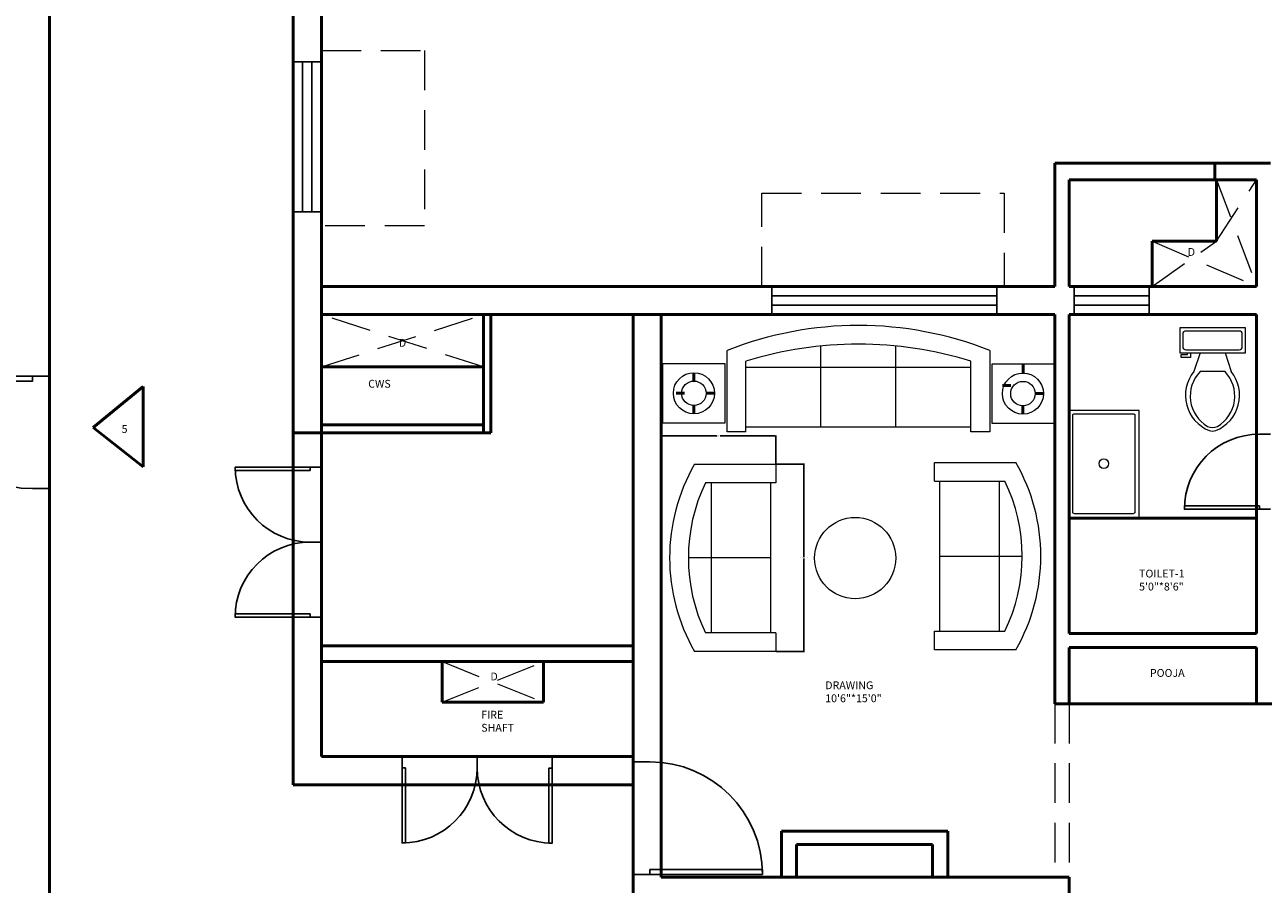
# Model space of a CAD drawing. Units: inches. Extents: x 291 to 2631, y 456 to 2623.
# Tile 18 of 22: x 1974 to 2370, y 1845 to 2120. Entities that reach past the tile are written whole.
import ezdxf

# ---------------------------------------------------------------- set-up
doc = ezdxf.new("R2010")
doc.units = ezdxf.units.IN
doc.linetypes.add('DASHED', pattern=[19.05, 12.7, -6.35])
for name, color, linetype, lineweight in [('A-ANNO-DIMS', 2, 'Continuous', 18), ('A-ANNO-TEXT', 3, 'Continuous', 25), ('A-AREA-IDEN', 7, 'Continuous', 25), ('A-DOOR', 3, 'Continuous', 25), ('A-FLOR-FIXT', 9, 'Continuous', 18), ('A-FLOR-OVHD', 1, 'DASHED', 18), ('A-FURN', 8, 'Continuous', 18), ('A-GLAZ', 4, 'Continuous', 25), ('A-WALL', 7, 'Continuous', 50)]:
    doc.layers.add(name, color=color, linetype=linetype, lineweight=lineweight)
doc.styles.get("Standard").update_dxf_attribs({"font": 'arial.ttf'})
doc.dimstyles.get("Standard").update_dxf_attribs({"dimtxt": 0.18, "dimasz": 0.18, "dimexe": 0.18, "dimexo": 0.0625, "dimgap": 0.09, "dimtad": 0, "dimtih": 1, "dimtoh": 1, "dimdec": 4, "dimzin": 0, "dimdsep": 46, "dimtxsty": 'Standard', "dimcen": 0.09, "dimadec": 0, "dimazin": 0, "dimtfac": 1, "dimtdec": 4, "dimtofl": 0, "dimtmove": 0, "dimatfit": 3, "dimfxl": 1, "dimtolj": 1, "dimtzin": 0, "dimarcsym": 0})

# ---------------------------------------------------------------- blocks, each defined once
blk = doc.blocks.new('*U2')
for p, q in [((0, 0), (0, -6)), ((40, 0), (40, -6))]:
    blk.add_line(p, q)
blk.add_lwpolyline([(0, 0), (0, 40), (1.75, 40), (1.75, 0)], close=True)
blk.add_arc((0, 0), 40, 0, 90)
blk = doc.blocks.new('Sofa - Roundback 7 ft.')
for p, q in [((-12.00002, -32.4421), (-12.00003, -6.5971)), ((11.99997, -32.4421), (11.99998, -6.5971)), ((-36.000027, -34), (-36.000027, -11.4696)), ((35.99998, -34), (35.99998, -11.4696)), ((-35.999844, -13.3819), (35.9998, -13.3819)), ((-36.000027, -32.4421), (35.99998, -32.4421))]:
    blk.add_line(p, q)
for points in [[(-36.000027, -34), (-42.000027, -34), (-42.000027, -8)], [(41.99998, -8), (41.99998, -34), (35.99998, -34)]]:
    blk.add_lwpolyline(points)
for centre, radius, start, end in [((0, -114.25), 114.25, 68.43141, 111.5686), ((-0.00001, -127.1968), 121.1968, 72.72033, 107.2797)]:
    blk.add_arc(centre, radius, start, end)
blk = doc.blocks.new('Sofa - Roundback Loveseat 5 ft.')
for p, q in [((0, -32.44198), (0, -5.99998)), ((-24, -33.99998), (-24, -11.46958)), ((24.00004, -33.99998), (24.00004, -11.46958)), ((-23.9998, -13.38178), (23.99986, -13.38178)), ((-24, -32.44198), (24.00004, -32.44198))]:
    blk.add_line(p, q)
for points in [[(-24, -33.99998), (-30, -33.99998), (-30, -7.99998)], [(30.00004, -7.99998), (30.00004, -33.99998), (24.00004, -33.99998)]]:
    blk.add_lwpolyline(points)
for centre, radius, start, end in [((0, -60.24998), 60.24998, 60.13715, 119.8628), ((0, -61.38438), 55.38444, 64.32083, 115.6792)]:
    blk.add_arc(centre, radius, start, end)
blk = doc.blocks.new('Toilet - top')
for p, q in [((9.5, -6), (9.5, -2)), ((-10, -8.5), (-8, -8.5)), ((-10, -9.5), (-10, -8.5)), ((-7, -9.5), (-10, -9.5)), ((-8, -8.5), (-8, -8)), ((-7, -8), (-7, -9.5)), ((-4, -8), (-6, -14)), ((4, -8), (6, -14)), ((4, -14), (-4, -14))]:
    blk.add_line(p, q)
blk.add_lwpolyline([(10.5, -8), (10.5, 0), (-10.5, 0), (-10.5, -8)], close=True)
for points in [[(-9.5, -2), (-9.5, -6)], [(8.5, -1), (-8.5, -1)], [(-8.5, -7), (8.5, -7)]]:
    blk.add_lwpolyline(points)
for centre, radius, start, end in [((-8.62, -1.88), 0.884, 81.8699, 188.1301), ((8.62, -1.88), 0.884, 351.8699, 98.1301), ((-8.62, -6.12), 0.884, 171.8699, 278.1301), ((8.62, -6.12), 0.884, 261.8699, 8.1301), ((3.52, -21.58), 12.17, 141.4691, 247.9714), ((4.2, -21.82), 11.33, 136.3677, 238.9468), ((-3.52, -21.58), 12.17, 292.0284, 38.5307), ((-4.2, -21.82), 11.33, 301.053, 43.6321), ((0, -27.88), 4, 245.7318, 294.2682), ((0, -29), 4, 254.8605, 285.1395)]:
    blk.add_arc(centre, radius, start, end)
blk = doc.blocks.new('WIN-1800')
for p, q in [((0, 9), (72, 9)), ((0, 0), (0, 9)), ((72, 9), (72, 0)), ((0, 6), (72, 6)), ((72, 3), (0, 3)), ((72, 0), (0, 0))]:
    blk.add_line(p, q)
blk = doc.blocks.new('WIN-1200')
for p, q in [((0, 0), (0, 48)), ((0, 48), (9, 48)), ((3, 0), (3, 48)), ((6, 48), (6, 0)), ((9, 48), (9, 0)), ((9, 0), (0, 0))]:
    blk.add_line(p, q)
blk = doc.blocks.new('WIN-600')
for p, q in [((24, 9), (0, 9)), ((0, 9), (0, 0)), ((24, 0), (24, 9)), ((24, 6), (0, 6)), ((0, 3), (24, 3)), ((0, 0), (24, 0))]:
    blk.add_line(p, q)
blk = doc.blocks.new('*D36')
at = {"layer": 'A-ANNO-DIMS', "color": 0, "lineweight": -2, "transparency": 16777216}
for p, q in [((2213.97, 1979.33), (2223.09, 1979.33)), ((2222.91, 1979.15), (2222.91, 1949.51)), ((2222.91, 1919.51), (2222.91, 1949.15)), ((2213.97, 1919.33), (2223.09, 1919.33))]:
    blk.add_line(p, q, dxfattribs=at)
at = {"layer": 'A-ANNO-DIMS', "color": 0, "transparency": 16777216}
for points in [[(2222.88, 1979.15), (2222.94, 1979.15), (2222.91, 1979.33)], [(2222.88, 1919.51), (2222.94, 1919.51), (2222.91, 1919.33)]]:
    blk.add_solid(points, dxfattribs=at)
at = {"layer": 'DEFPOINTS', "color": 0, "transparency": 16777216}
for p in [(2213.91, 1979.33), (2222.91, 1979.33), (2213.91, 1919.33)]:
    blk.add_point(p, dxfattribs=at)
at = {"layer": 'A-ANNO-DIMS', "color": 0, "transparency": 16777216, "insert": (2222.91, 1949.33), "char_height": 0.18, "attachment_point": 5}
blk.add_mtext('\\A1;LOVESEAT 5 FT 60 TYP.', dxfattribs=at)
blk = doc.blocks.new('*D37')
at = {"layer": 'A-ANNO-DIMS', "color": 0, "lineweight": -2, "transparency": 16777216}
for p, q in [((2177.24, 1979.39), (2177.24, 1988.51)), ((2177.42, 1988.33), (2195.05, 1988.33)), ((2213.73, 1988.33), (2196.1, 1988.33)), ((2213.91, 1979.39), (2213.91, 1988.51))]:
    blk.add_line(p, q, dxfattribs=at)
at = {"layer": 'A-ANNO-DIMS', "color": 0, "transparency": 16777216}
for points in [[(2177.42, 1988.36), (2177.42, 1988.3), (2177.24, 1988.33)], [(2213.73, 1988.36), (2213.73, 1988.3), (2213.91, 1988.33)]]:
    blk.add_solid(points, dxfattribs=at)
at = {"layer": 'DEFPOINTS', "color": 0, "transparency": 16777216}
for p in [(2177.24, 1988.33), (2177.24, 1979.33), (2213.91, 1979.33)]:
    blk.add_point(p, dxfattribs=at)
at = {"layer": 'A-ANNO-DIMS', "color": 0, "transparency": 16777216, "insert": (2195.57, 1988.33), "char_height": 0.18, "attachment_point": 5}
blk.add_mtext('\\A1;37 TYP.', dxfattribs=at)

msp = doc.modelspace()

# ---------------------------------------------------------------- linework, layer by layer
at = {"layer": 'A-FLOR-OVHD'}
for p, q in [((2068.49, 2111.63), (2101.5, 2111.63)), ((2101.5, 2111.63), (2101.5, 2055.54)), ((2354.93, 2050.69), (2367.71, 2070.31)), ((2354.93, 2070.31), (2367.71, 2036.14)), ((2209.38, 2036.14), (2209.38, 2065.98)), ((2209.38, 2065.98), (2286.98, 2065.98)), ((2286.98, 2065.98), (2286.98, 2036.14)), ((2101.5, 2055.54), (2068.49, 2055.54)), ((2334.27, 2050.69), (2367.71, 2036.14)), ((2334.27, 2036.14), (2354.93, 2050.69)), ((2068.49, 2010.39), (2120.33, 2027.14)), ((2120.33, 2010.39), (2068.49, 2027.14)), ((2107.13, 1916.12), (2139.59, 1903.11)), ((2107.13, 1903.11), (2139.59, 1916.12)), ((2303.21, 1902.64), (2303.21, 1847.14)), ((2307.71, 1902.64), (2307.71, 1847.14))]:
    msp.add_line(p, q, dxfattribs=at)
at = {"layer": 'A-FURN'}
for points in [[(2177.8, 2011.54), (2197.59, 2011.54), (2197.59, 1992.4), (2177.8, 1992.4)], [(2283.07, 2011.44), (2302.86, 2011.44), (2302.86, 1992.31), (2283.07, 1992.31)], [(2307.71, 1962.04), (2330.17, 1962.04), (2330.17, 1996.48), (2307.71, 1996.48)]]:
    msp.add_lwpolyline(points, close=True, dxfattribs=at)
msp.add_lwpolyline([(2309.43, 1995.44), (2328.25, 1995.44, -0.414214), (2328.75, 1994.94), (2328.75, 1963.95, -0.414214), (2328.25, 1963.45), (2309.43, 1963.45, -0.414214), (2308.93, 1963.95), (2308.93, 1994.94, -0.414214)], format="xyb", close=True, dxfattribs=at)
for centre, radius in [((2187.69, 2001.97), 6.58), ((2187.69, 2001.97), 3.91), ((2292.96, 2001.87), 6.58), ((2292.96, 2001.87), 3.91), ((2318.84, 1979.45), 1.54), ((2239.29, 1949.24), 13)]:
    msp.add_circle(centre, radius, dxfattribs=at)
at = {"layer": 'A-WALL'}
for p, q in [((1981.49, 2156.24), (1981.49, 1804.93)), ((2059.49, 2156.24), (2059.49, 1916.04)), ((2068.49, 2156.24), (2068.49, 1916.12)), ((2303.21, 2036.14), (2303.21, 2075.57)), ((2303.21, 2075.57), (2372.21, 2075.57)), ((2354.39, 2075.57), (2354.39, 2070.31)), ((2307.71, 2036.14), (2307.71, 2070.31)), ((2307.71, 2070.31), (2367.71, 2070.31)), ((2354.93, 2070.31), (2354.93, 2050.69)), ((2367.71, 2070.31), (2367.71, 2036.14)), ((2354.93, 2050.69), (2334.27, 2050.69)), ((2334.27, 2050.69), (2334.27, 2036.14)), ((2068.49, 2036.14), (2303.21, 2036.14)), ((2307.71, 2036.14), (2367.71, 2036.14)), ((2068.49, 2027.14), (2303.21, 2027.14)), ((2120.33, 1989.28), (2120.33, 2027.14)), ((2122.76, 2027.14), (2122.76, 1989.28)), ((2168.21, 2027.14), (2168.21, 1876.71)), ((2177.21, 2027.14), (2177.21, 1876.71)), ((2303.21, 2027.14), (2303.21, 1902.64)), ((2307.71, 2027.14), (2307.71, 1925.14)), ((2307.71, 2027.14), (2367.71, 2027.14)), ((2367.71, 2027.14), (2367.71, 1925.14)), ((2367.71, 2027.14), (2367.71, 1925.14)), ((2068.49, 2010.39), (2120.33, 2010.39)), ((2293.02, 2011.04), (2293.02, 2008.37)), ((2187.69, 2008.55), (2187.69, 2005.88)), ((2011.49, 2004.11), (1995.51, 1991.06)), ((2011.49, 2004.11), (2011.49, 1978.48)), ((2181.99, 2001.97), (2184.67, 2001.97)), ((2191.6, 2001.97), (2194.27, 2001.97)), ((2286.44, 2004.46), (2289.11, 2004.46)), ((2296.87, 2001.87), (2299.54, 2001.87)), ((2187.69, 1998.06), (2187.69, 1995.39)), ((2292.96, 1997.97), (2292.96, 1995.3)), ((1995.51, 1991.06), (2011.49, 1978.48)), ((2068.49, 1989.28), (2059.49, 1989.28)), ((2068.49, 1991.9), (2120.33, 1991.9)), ((2122.76, 1989.28), (2068.49, 1989.28)), ((2307.71, 1962.04), (2367.71, 1962.04)), ((2307.71, 1925.14), (2367.71, 1925.14)), ((2068.49, 1921.18), (2168.21, 1921.18)), ((2307.71, 1920.64), (2367.71, 1920.64)), ((2307.71, 1920.64), (2307.71, 1902.64)), ((2367.71, 1920.64), (2367.71, 1902.64)), ((2367.71, 1920.64), (2367.71, 1902.64)), ((2059.49, 1916.04), (2059.49, 1876.71)), ((2068.49, 1916.12), (2068.49, 1885.71)), ((2068.49, 1916.12), (2168.21, 1916.12)), ((2107.13, 1916.12), (2107.13, 1903.11)), ((2139.59, 1903.11), (2139.59, 1916.12)), ((2107.13, 1903.11), (2139.59, 1903.11)), ((2367.71, 1902.64), (2303.21, 1902.64)), ((2367.71, 1902.64), (2405.25, 1902.64)), ((2068.49, 1885.71), (2168.21, 1885.71)), ((2059.49, 1876.71), (2168.21, 1876.71)), ((2168.21, 1876.71), (2168.21, 1650.64)), ((2177.21, 1876.71), (2177.21, 1847.14)), ((2215.75, 1847.14), (2215.75, 1861.82)), ((2215.75, 1861.82), (2268.97, 1861.82)), ((2268.97, 1861.82), (2268.97, 1847.14)), ((2220.49, 1847.14), (2220.49, 1857.57)), ((2220.49, 1857.57), (2264.03, 1857.57)), ((2264.03, 1857.57), (2264.03, 1847.14)), ((2177.21, 1847.14), (2307.71, 1847.14)), ((2307.71, 1847.14), (2307.71, 1837.02))]:
    msp.add_line(p, q, dxfattribs=at)

# ---------------------------------------------------------------- block references
at = {"layer": 'A-DOOR'}
for p, xscale, yscale, zscale, rotation in [((1976.09, 2007.47), -0.9, 0.9, 0.9, 90), ((2368.61, 1964.89), 0.6, 0.6, 0.6, 90.00000000000003), ((2064.94, 1978.34), -0.6, 0.6, 0.6, 90), ((2064.89, 1930.34), 0.6, 0.6, 0.6, 90.00000000000003), ((2094.35, 1882.11), -0.6, 0.6, 0.6, 180), ((2142.35, 1882.06), 0.6, 0.6, 0.6, 180), ((2173.61, 1848.02), -0.9, 0.9, 0.9, 270)]:
    msp.add_blockref('*U2', p, dxfattribs=dict(at, xscale=xscale, yscale=yscale, zscale=zscale, rotation=rotation))
at = {"layer": 'A-FLOR-FIXT'}
msp.add_blockref('Toilet - top', (2353.62, 2022.89), dxfattribs=at)
at = {"layer": 'A-FURN'}
msp.add_blockref('Sofa - Roundback 7 ft.', (2240.34, 2023.67), dxfattribs=at)
for p, rotation in [((2179.91, 1949.33), 90), ((2298.69, 1949.87), 270.0000000000006)]:
    msp.add_blockref('Sofa - Roundback Loveseat 5 ft.', p, dxfattribs=dict(at, rotation=rotation))
at = {"layer": 'A-GLAZ'}
for name, p in [('WIN-1200', (2059.49, 2059.97)), ('WIN-1800', (2212.65, 2027.14))]:
    msp.add_blockref(name, p, dxfattribs=at)
at = {"layer": 'A-GLAZ', "rotation": 180}
msp.add_blockref('WIN-600', (2333.33, 2036.14), dxfattribs=at)

# ---------------------------------------------------------------- texts
at = {"layer": 'A-ANNO-TEXT', "char_height": 2.5, "attachment_point": 1}
for s, width, insert in [('D', 2.135, (2345.69, 2048.44)), ('D', 2.1199, (2093.29, 2019.36)), ('CWS', 27.3646, (2083.48, 2006.26)), ('5', 6.4727, (2004.59, 1991.78)), ('D', 2.4925, (2122.59, 1912.61))]:
    msp.add_mtext_dynamic_manual_height_columns(s, width=width, gutter_width=12.5, heights=[0], dxfattribs=dict(at, insert=insert))
at = {"layer": 'A-AREA-IDEN', "char_height": 2.5, "attachment_point": 1}
for s, width, insert in [('TOILET-1\\P5\'0"*8\'6"', 43.4526, (2330.12, 1945.54)), ('POOJA', 30.0751, (2333.59, 1913.74)), ('DRAWING\\P10\'6"*15\'0"', 51.2299, (2229.7, 1909.79)), ('FIRE\\PSHAFT', 32.6186, (2119.65, 1900.37))]:
    msp.add_mtext_dynamic_manual_height_columns(s, width=width, gutter_width=12.5, heights=[0], dxfattribs=dict(at, insert=insert))

# ---------------------------------------------------------------- dimensions: what is measured, and where the dimension line sits
at = {"layer": 'A-ANNO-DIMS'}
for base, p1, p2, angle, text, picture, middle in [((2177.24, 1988.33), (2213.91, 1979.33), (2177.24, 1979.33), 180, '<> TYP.', '*D37', (2195.57, 1988.33)), ((2222.91, 1979.33), (2213.91, 1919.33), (2213.91, 1979.33), 90, 'LOVESEAT 5 FT <> TYP.', '*D36', (2222.91, 1949.33))]:
    dim = msp.add_linear_dim(base=base, p1=p1, p2=p2, angle=angle, text=text, dimstyle='Standard', override={"dimdec": 0, "dimlfac": 1, "dimrnd": 0, "dimzin": 0, "dimdsep": 46, "dimlunit": 2}, dxfattribs=at)
    dim.commit()
    dim.dimension.update_dxf_attribs({"geometry": picture, "text_midpoint": middle})

doc.saveas('drawing.dxf')
